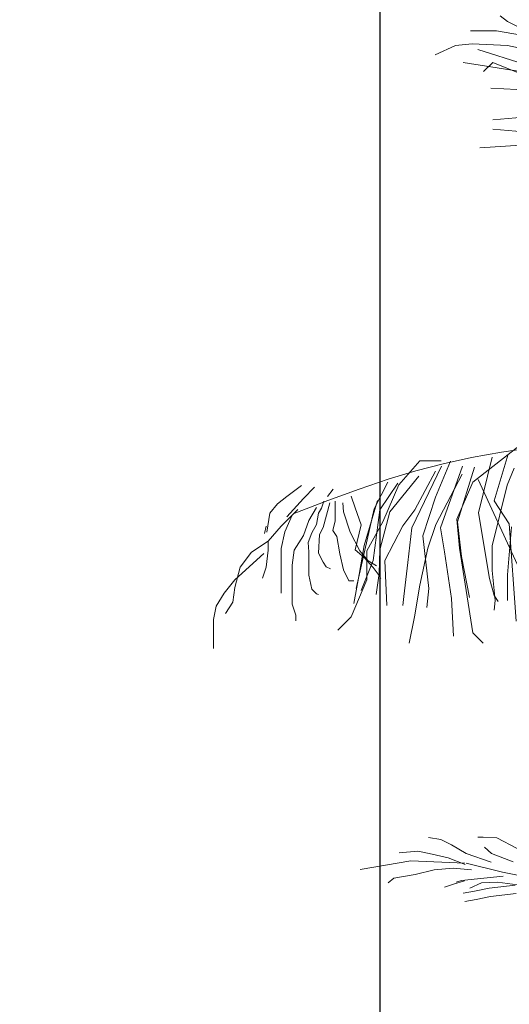
# Model space of a CAD drawing. Units: millimetres. Extents: x 595116 to 630915, y 909473 to 920225.
# Tile 55 of 134: x 629588.98 to 629595.73, y 919288.02 to 919301.58. Entities that reach past the tile are written whole.
import ezdxf

# ---------------------------------------------------------------- set-up
doc = ezdxf.new("R2010")
doc.units = ezdxf.units.MM
doc.layers.add('Dimension', color=3, linetype='Continuous', lineweight=18)
doc.layers.add('L-PLNT', color=85, linetype='Continuous', lineweight=13)
doc.styles.get("Standard").update_dxf_attribs({"font": 'arial.ttf'})
doc.dimstyles.new('ISO-25', dxfattribs={"dimtxt": 9, "dimasz": 6, "dimexe": 1.25, "dimexo": 0.625, "dimtad": 1, "dimlunit": 4, "dimtxsty": 'Standard', "dimcen": 2.5, "dimadec": 0, "dimazin": 0, "dimtfac": 1, "dimtmove": 0, "dimatfit": 3, "dimfxl": 1, "dimarcsym": 0})

# ---------------------------------------------------------------- blocks, each defined once
blk = doc.blocks.new('A$C4FB75ABC')
for p, q in [((1.0518, 3.8421), (1.079, 3.8217)), ((1.079, 3.8217), (1.1199, 3.8012)), ((0.9428, 3.7876), (1.0382, 3.7876)), ((1.0382, 3.7876), (1.2698, 3.7467)), ((0.8133, 3.6991), (0.8883, 3.7331)), ((0.8883, 3.7331), (0.9496, 3.7399)), ((0.9496, 3.7399), (1.079, 3.7331)), ((1.079, 3.7331), (1.1812, 3.7127)), ((0.97, 3.7195), (1.1403, 3.665)), ((0.9155, 3.6718), (1.1267, 3.6378)), ((1.0245, 3.6718), (0.9905, 3.6378)), ((1.1403, 3.6242), (1.0245, 3.6718)), ((1.0177, 3.5765), (1.1608, 3.5697)), ((1.0245, 3.4608), (1.1744, 3.4744)), ((1.0245, 3.4267), (1.1812, 3.4131)), ((0.9768, 3.3586), (1.3107, 3.379)), ((1.1746, 2.3061), (0.9513, 2.1315)), ((1.0564, 2.241), (0.9464, 2.2213)), ((1.1767, 2.2586), (1.0564, 2.241)), ((0.7572, 2.2091), (0.6795, 2.1218)), ((0.8348, 2.2091), (0.7572, 2.2091)), ((0.8699, 2.2079), (0.8151, 2.0766)), ((0.9464, 2.2213), (0.8429, 2.1986)), ((1.0231, 2.2224), (0.972, 2.0182)), ((1.0815, 2.2334), (1.0304, 2.062)), ((0.7422, 2.1723), (0.6405, 2.1416)), ((0.837, 2.1896), (0.7276, 1.9635)), ((0.8151, 2.1714), (0.7385, 2.0291)), ((0.8429, 2.1986), (0.7422, 2.1723)), ((0.9137, 2.1896), (0.8334, 1.9635)), ((0.9575, 2.186), (0.8954, 1.9854)), ((1.1034, 2.1823), (1.0779, 2.1203)), ((0.6405, 2.1416), (0.5342, 2.1057)), ((0.7531, 2.1531), (0.6473, 2.0218)), ((0.9125, 2.1606), (0.8154, 1.9763)), ((1.2522, 1.53), (0.9707, 2.1412)), ((0.2683, 2.0784), (0.3228, 2.1193)), ((0.3296, 2.0716), (0.3705, 2.1125)), ((0.4182, 2.0784), (0.4386, 2.1057)), ((0.5342, 2.1057), (0.4195, 2.0639)), ((0.64, 2.1313), (0.5889, 2.0328)), ((0.6765, 2.1276), (0.6108, 2.0291)), ((0.6795, 2.1218), (0.6213, 1.986)), ((0.9513, 2.1315), (0.8931, 1.9957)), ((1.0779, 2.1203), (1.0231, 1.8978)), ((0.2342, 2.0512), (0.2683, 2.0784)), ((0.2683, 2.0035), (0.3296, 2.0716)), ((0.4195, 2.0639), (0.2927, 2.0154)), ((0.4049, 2.0609), (0.3966, 2.0361)), ((0.4463, 2.0609), (0.4463, 1.9892)), ((0.505, 2.0802), (0.5196, 2.0364)), ((0.6018, 2.0636), (0.5533, 1.8986)), ((0.8151, 2.0766), (0.7677, 1.9343)), ((1.0304, 2.062), (1.0852, 1.9781)), ((0.207, 2.0172), (0.2342, 2.0512)), ((0.3092, 2.0308), (0.2479, 1.9695)), ((0.3773, 2.0376), (0.3501, 1.9899)), ((0.3966, 2.0361), (0.3855, 2.0168)), ((0.427, 2.0554), (0.4021, 1.9643)), ((0.4739, 2.0554), (0.4767, 2.0223)), ((0.5196, 2.0364), (0.5415, 1.9744)), ((0.5889, 2.0328), (0.5232, 1.741)), ((0.6108, 2.0291), (0.5853, 1.8431)), ((0.7385, 2.0291), (0.6947, 1.9708)), ((0.195, 1.9478), (0.207, 2.0172)), ((0.2887, 2.0103), (0.2615, 1.9491)), ((0.3501, 1.9899), (0.3296, 1.9354)), ((0.3855, 2.0168), (0.3773, 1.9754)), ((0.4463, 1.9892), (0.438, 1.9533)), ((0.4767, 2.0223), (0.5015, 1.9478)), ((0.6473, 2.0218), (0.6108, 1.8833)), ((0.8931, 1.9957), (0.9028, 1.8889)), ((0.972, 2.0182), (1.0122, 1.7775)), ((0.1865, 1.9422), (0.1934, 1.9695)), ((0.2479, 1.9695), (0.2002, 1.915)), ((0.3773, 1.9754), (0.3607, 1.945)), ((0.4021, 1.9643), (0.3883, 1.9395)), ((0.438, 1.9533), (0.4518, 1.9312)), ((0.5415, 1.9744), (0.5196, 1.8833)), ((0.6213, 1.986), (0.563, 1.8792)), ((0.6947, 1.9708), (0.629, 1.8431)), ((0.7276, 1.9635), (0.713, 1.8358)), ((0.8154, 1.9763), (0.7863, 1.8889)), ((0.8334, 1.9635), (0.848, 1.876)), ((0.8954, 1.9854), (0.91, 1.8577)), ((1.0939, 1.9669), (1.0786, 1.7905)), ((1.0852, 1.9781), (1.1107, 1.6207)), ((0.2615, 1.9491), (0.2479, 1.8878)), ((0.3296, 1.9354), (0.2956, 1.881)), ((0.3607, 1.945), (0.3469, 1.9091)), ((0.3883, 1.9395), (0.3855, 1.8705)), ((0.4518, 1.9312), (0.4629, 1.8677)), ((0.5015, 1.9478), (0.5374, 1.8788)), ((0.7677, 1.9343), (0.7896, 1.741)), ((0.2002, 1.915), (0.1389, 1.8742)), ((0.2002, 1.881), (0.1934, 1.8197)), ((0.2002, 1.915), (0.2002, 1.881)), ((0.2479, 1.8878), (0.2479, 1.8061)), ((0.2956, 1.881), (0.2887, 1.8265)), ((0.3469, 1.9091), (0.3497, 1.876)), ((0.5196, 1.8833), (0.5524, 1.8541)), ((0.5533, 1.8986), (0.5339, 1.7919)), ((0.563, 1.8792), (0.563, 1.7725)), ((0.6108, 1.8833), (0.6072, 1.7957)), ((0.7863, 1.8889), (0.7572, 1.7531)), ((0.9028, 1.8889), (0.9513, 1.5785)), ((1.0231, 1.8978), (1.0231, 1.8067)), ((0.1844, 1.8695), (0.0777, 1.7725)), ((0.1389, 1.8742), (0.098, 1.8197)), ((0.3497, 1.876), (0.3497, 1.8512)), ((0.3497, 1.8512), (0.3497, 1.7904)), ((0.3855, 1.8705), (0.4021, 1.8374)), ((0.4629, 1.8677), (0.4767, 1.8098)), ((0.5374, 1.8788), (0.5678, 1.8429)), ((0.5853, 1.8431), (0.5415, 1.7337)), ((0.5524, 1.8541), (0.5853, 1.8176)), ((0.629, 1.8431), (0.6363, 1.679)), ((0.848, 1.876), (0.8735, 1.7045)), ((0.91, 1.8577), (0.9392, 1.7082)), ((0.098, 1.8197), (0.0775, 1.7448)), ((0.1934, 1.8197), (0.1797, 1.7788)), ((0.2887, 1.8265), (0.2887, 1.7516)), ((0.4021, 1.8374), (0.4132, 1.8208)), ((0.4132, 1.8208), (0.4297, 1.8125)), ((0.4767, 1.8098), (0.496, 1.7684)), ((0.5678, 1.8429), (0.5982, 1.8236)), ((0.5853, 1.8176), (0.6072, 1.7884)), ((0.713, 1.8358), (0.6984, 1.7118)), ((0.0777, 1.7725), (0.0388, 1.724)), ((0.2479, 1.8061), (0.2479, 1.7448)), ((0.3497, 1.7904), (0.3607, 1.738)), ((0.563, 1.7725), (0.5048, 1.6367)), ((0.5339, 1.7919), (0.5145, 1.6852)), ((0.6072, 1.7957), (0.5962, 1.7191)), ((0.6072, 1.7884), (0.6144, 1.7775)), ((1.0122, 1.7775), (1.0304, 1.7155)), ((1.0231, 1.8067), (1.0341, 1.6973)), ((1.0786, 1.7905), (1.0786, 1.6973)), ((0.0775, 1.7448), (0.0707, 1.6903)), ((0.2479, 1.7448), (0.2479, 1.7243)), ((0.2887, 1.7516), (0.2887, 1.6835)), ((0.3607, 1.738), (0.3773, 1.7214)), ((0.496, 1.7684), (0.5153, 1.7684)), ((0.7572, 1.7531), (0.7377, 1.6367)), ((0.7896, 1.741), (0.7823, 1.6717)), ((0.0388, 1.724), (0.0097, 1.6755)), ((0.3773, 1.7214), (0.3855, 1.7187)), ((0.6984, 1.7118), (0.6947, 1.679)), ((0.8735, 1.7045), (0.8808, 1.566)), ((1.0304, 1.7155), (1.045, 1.6936)), ((0.0097, 1.6755), (0, 1.627)), ((0.0707, 1.6903), (0.0435, 1.6494)), ((0.2887, 1.6835), (0.3024, 1.6426)), ((1.0341, 1.6973), (1.0304, 1.6608)), ((0, 1.627), (0, 1.5494)), ((0.3024, 1.6426), (0.3024, 1.6222)), ((0.5048, 1.6367), (0.4562, 1.5882)), ((0.7377, 1.6367), (0.7183, 1.5397)), ((0.9513, 1.5785), (0.9901, 1.5397)), ((0, 1.5494), (0, 1.5203)), ((0.8346, 0.8198), (0.7888, 0.827)), ((0.8736, 0.7996), (0.8346, 0.8198)), ((0.9273, 0.7678), (0.8736, 0.7996)), ((0.9891, 0.8277), (0.9703, 0.828)), ((1.04, 0.8252), (0.9891, 0.8277)), ((1.1149, 0.7864), (1.04, 0.8252)), ((0.7503, 0.7767), (0.6814, 0.7711)), ((0.7912, 0.768), (0.7503, 0.7767)), ((0.8615, 0.7523), (0.7912, 0.768)), ((1.0187, 0.737), (0.9273, 0.7678)), ((1.0204, 0.7689), (0.9943, 0.7918)), ((1.0992, 0.7376), (1.0204, 0.7689)), ((0.7236, 0.7411), (0.5379, 0.7092)), ((0.9219, 0.7334), (0.7236, 0.7411)), ((0.9235, 0.7285), (0.8615, 0.7523)), ((1.0599, 0.6997), (0.9265, 0.7333)), ((0.7393, 0.6917), (0.6621, 0.678)), ((0.8101, 0.7087), (0.7393, 0.6917)), ((0.879, 0.7143), (0.8101, 0.7087)), ((0.9462, 0.7085), (0.879, 0.7143)), ((1.1712, 0.6779), (1.0599, 0.6997)), ((0.6621, 0.678), (0.6405, 0.6602)), ((0.8811, 0.6557), (0.847, 0.6449)), ((0.9209, 0.6684), (0.8811, 0.6557)), ((0.9095, 0.6697), (0.8898, 0.6634)), ((1.0623, 0.6856), (0.9095, 0.6697)), ((0.9832, 0.6605), (0.9403, 0.6414)), ((1.0423, 0.6629), (0.9832, 0.6605)), ((1.1074, 0.6526), (1.011, 0.6408)), ((1.1159, 0.6537), (1.0423, 0.6629)), ((0.9581, 0.6302), (0.9165, 0.6232)), ((1.011, 0.6408), (0.9581, 0.6302)), ((1.1106, 0.6216), (1.016, 0.61)), ((0.9632, 0.5994), (0.9216, 0.5925)), ((1.016, 0.61), (0.9632, 0.5994))]:
    blk.add_line(p, q)
blk = doc.blocks.new('*D210')
at = {"layer": 'Defpoints', "color": 0, "transparency": 16777216}
for p in [(629586.227, 919310.123), (629593.946, 919310.123), (629586.227, 919258.662)]:
    blk.add_point(p, dxfattribs=at)
at = {"layer": 'Dimension', "color": 0, "lineweight": -2, "transparency": 16777216}
for p, q in [((629593.946, 919310.123), (629593.946, 919449.69)), ((629586.852, 919310.123), (629595.196, 919310.123)), ((629593.946, 919264.662), (629593.946, 919304.123)), ((629586.852, 919258.662), (629595.196, 919258.662))]:
    blk.add_line(p, q, dxfattribs=at)
at = {"layer": 'Dimension', "color": 0, "transparency": 16777216}
for points in [[(629592.946, 919304.123), (629594.946, 919304.123), (629593.946, 919310.123)], [(629592.946, 919264.662), (629594.946, 919264.662), (629593.946, 919258.662)]]:
    blk.add_solid(points, dxfattribs=at)
at = {"layer": 'Dimension', "color": 0, "transparency": 16777216, "insert": (629588.662, 919382.907), "char_height": 9, "attachment_point": 5, "rotation": 90}
blk.add_mtext('CANOPY 4\'-3 1/2" TYP.', dxfattribs=at)
blk = doc.blocks.new('*D216')
at = {"layer": 'Defpoints', "color": 0, "transparency": 16777216}
for p in [(629743.541, 919411.928), (629505.041, 919411.828), (629743.541, 918832.378)]:
    blk.add_point(p, dxfattribs=at)
at = {"layer": 'Dimension', "color": 0, "lineweight": -2, "transparency": 16777216}
for p, q in [((629505.041, 919411.203), (629505.041, 918831.128)), ((629743.541, 919411.303), (629743.541, 918831.128)), ((629511.041, 918832.378), (629737.541, 918832.378))]:
    blk.add_line(p, q, dxfattribs=at)
at = {"layer": 'Dimension', "color": 0, "transparency": 16777216}
for points in [[(629511.041, 918833.378), (629511.041, 918831.378), (629505.041, 918832.378)], [(629737.541, 918833.378), (629737.541, 918831.378), (629743.541, 918832.378)]]:
    blk.add_solid(points, dxfattribs=at)
at = {"layer": 'Dimension', "color": 0, "transparency": 16777216, "insert": (629624.291, 918837.656), "char_height": 9, "attachment_point": 5}
blk.add_mtext('19\'-10 1/2"', dxfattribs=at)

msp = doc.modelspace()

# ---------------------------------------------------------------- block references
at = {"layer": 'L-PLNT', "xscale": 3.753413438031968, "yscale": 3.753413438031968, "zscale": 3.753413438031968}
msp.add_blockref('A$C4FB75ABC', (629591.653, 919287.212), dxfattribs=at)

# ---------------------------------------------------------------- dimensions: what is measured, and where the dimension line sits
at = {"layer": 'Dimension'}
dim = msp.add_linear_dim(base=(629593.946, 919310.123), p1=(629586.227, 919258.662), p2=(629586.227, 919310.123), angle=90, text='CANOPY <> TYP.', dimstyle='ISO-25', override={"dimdec": 1, "dimlfac": 1, "dimrnd": 0, "dimzin": 1, "dimdsep": 46, "dimlunit": 4, "dimfrac": 2}, dxfattribs=at)
dim.commit()
dim.dimension.update_dxf_attribs({"geometry": '*D210', "text_midpoint": (629588.662, 919382.907)})
dim = msp.add_linear_dim(base=(629743.541, 918832.378), p1=(629505.041, 919411.828), p2=(629743.541, 919411.928), dimstyle='ISO-25', override={"dimdec": 1, "dimlfac": 1, "dimrnd": 0, "dimzin": 1, "dimdsep": 46, "dimlunit": 4, "dimfrac": 2}, dxfattribs=at)
dim.commit()
dim.dimension.update_dxf_attribs({"geometry": '*D216', "text_midpoint": (629624.291, 918837.656)})

doc.saveas('drawing.dxf')
